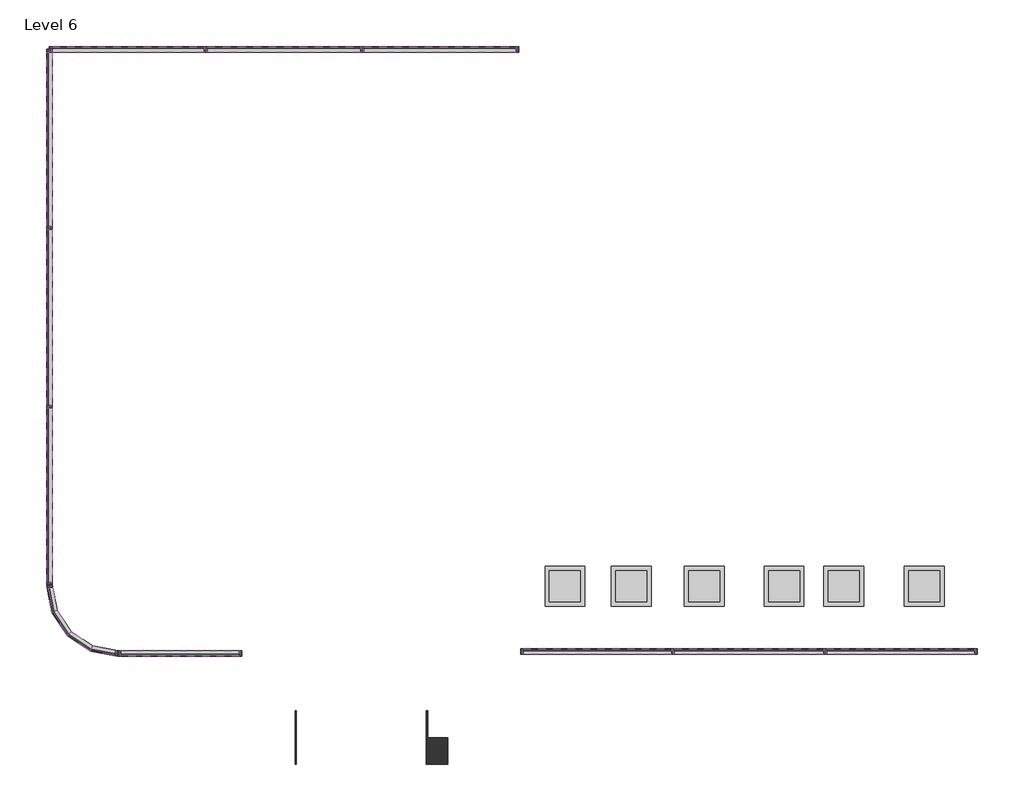
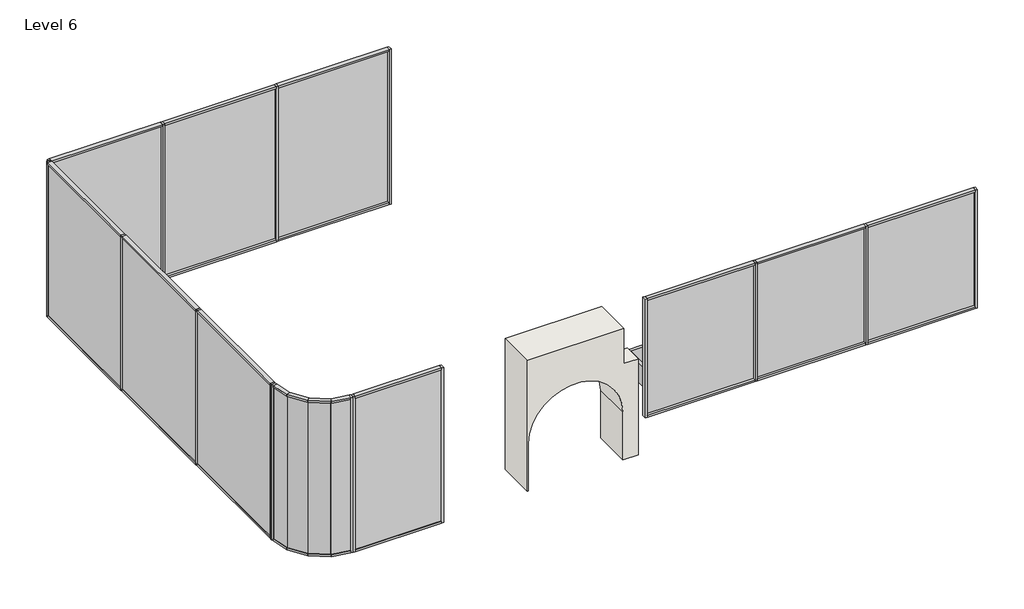
# One storey, incomplete: 44 members, 14 plates, 6 geographic elements, 1 wall.
"""IFC4 building model written with IfcOpenShell, lengths in millimetres."""

from ifc_helpers import new_model, si_unit, frame, origin, place, context, project, spatial, polyline, circle_curve, transform, mapped, element, save
from ifc_brep_helpers import plane_surface, revolved_surface, advanced_brep
from components import geographic_element_4c884dac, member_e5c989f4, member_5be86ab4, member_c6c1cc64, member_e826b105, member_eb03db27, member_3a1e0d67, member_7582bdd1, member_49f7f43a, member_78a27e2d, member_6a95fd14, member_1706ff29, member_70a47126, member_8659189c, member_4115b715, system_panel_glazed_8a9794be, system_panel_glazed_b9555dd7, system_panel_glazed_2aedba99, system_panel_glazed_5cb243be, system_panel_glazed_83a6671e, system_panel_glazed_ccff25ac, system_panel_glazed_ecbfc98a, system_panel_glazed_8a9bbf22, system_panel_glazed_1ec048b2

model = new_model("IFC4")

# Units and contexts
model_context = context("Model", 3, world=origin())
ifc_project = project(units=[si_unit("LENGTHUNIT", "METRE", prefix="MILLI")], contexts=[model_context])

# Site, building, storey
site = spatial("IfcSite", under=ifc_project)
building = spatial("IfcBuilding", under=site)
storey = spatial("IfcBuildingStorey", under=building, Name="Level 6", Elevation=12192.0)

# Geographic elements
placement = place(None, origin())
geographic_element_shape = geographic_element_4c884dac(model_context)
element("IfcGeographicElement", 1, ObjectType="Planter : 36\" x 36\"", at=placement, inside=storey, context=model_context, shape_type="MappedRepresentation", body=[
    mapped(geographic_element_shape, transform((3263.6150045, -1527.9908042, 11277.6), x_axis=(1.0, 0.0, 0.0), y_axis=(0.0, 1.0, 0.0), z_axis=(0.0, 0.0, 1.0))),
])
element("IfcGeographicElement", 2, ObjectType="Planter : 36\" x 36\"", at=placement, inside=storey, context=model_context, shape_type="MappedRepresentation", body=[
    mapped(geographic_element_shape, transform((1413.563121, -1527.9908042, 11277.6), x_axis=(1.0, 0.0, 0.0), y_axis=(0.0, 1.0, 0.0), z_axis=(0.0, 0.0, 1.0))),
])
element("IfcGeographicElement", 3, ObjectType="Planter : 36\" x 36\"", at=placement, inside=storey, context=model_context, shape_type="MappedRepresentation", body=[
    mapped(geographic_element_shape, transform((41.963121, -1527.9908042, 11277.6), x_axis=(1.0, 0.0, 0.0), y_axis=(0.0, 1.0, 0.0), z_axis=(0.0, 0.0, 1.0))),
])
element("IfcGeographicElement", 4, ObjectType="Planter : 36\" x 36\"", at=placement, inside=storey, context=model_context, shape_type="MappedRepresentation", body=[
    mapped(geographic_element_shape, transform((-1786.836879, -1527.9908042, 11277.6), x_axis=(1.0, 0.0, 0.0), y_axis=(0.0, 1.0, 0.0), z_axis=(0.0, 0.0, 1.0))),
])
element("IfcGeographicElement", 5, ObjectType="Planter : 36\" x 36\"", at=placement, inside=storey, context=model_context, shape_type="MappedRepresentation", body=[
    mapped(geographic_element_shape, transform((-3463.236879, -1527.9908042, 11277.6), x_axis=(1.0, 0.0, 0.0), y_axis=(0.0, 1.0, 0.0), z_axis=(0.0, 0.0, 1.0))),
])
element("IfcGeographicElement", 6, ObjectType="Planter : 36\" x 36\"", at=placement, inside=storey, context=model_context, shape_type="MappedRepresentation", body=[
    mapped(geographic_element_shape, transform((-4987.236879, -1527.9908042, 11277.6), x_axis=(1.0, 0.0, 0.0), y_axis=(0.0, 1.0, 0.0), z_axis=(0.0, 0.0, 1.0))),
])

# Members
member_shape = member_e5c989f4(model_context)
element("IfcMember", 7, ObjectType="Rectangular Mullion : 2.5\" x 5\" rectangular", at=placement, inside=storey, context=model_context, shape_type="MappedRepresentation", body=[
    mapped(member_shape, transform((-2507.8862511, -3028.3602909, 11201.4), x_axis=(1.0, 0.0, 0.0), y_axis=(0.0, -1.0, 0.0), z_axis=(0.0, 0.0, -1.0))),
])
element("IfcMember", 8, ObjectType="Rectangular Mullion : 2.5\" x 5\" rectangular", at=placement, inside=storey, context=model_context, shape_type="MappedRepresentation", body=[
    mapped(member_shape, transform((987.4643767, -3028.3602909, 11201.4), x_axis=(1.0, 0.0, 0.0), y_axis=(0.0, -1.0, 0.0), z_axis=(0.0, 0.0, -1.0))),
])
member_2_shape = member_5be86ab4(model_context)
element("IfcMember", 9, ObjectType="Rectangular Mullion : 2.5\" x 5\" rectangular", at=placement, inside=storey, context=model_context, shape_type="MappedRepresentation", body=[
    mapped(member_2_shape, transform((4482.8150045, -3028.3602909, 11201.4), x_axis=(1.0, 0.0, 0.0), y_axis=(0.0, -1.0, 0.0), z_axis=(0.0, 0.0, -1.0))),
])
element("IfcMember", 10, ObjectType="Rectangular Mullion : 2.5\" x 5\" rectangular", at=placement, inside=storey, context=model_context, shape_type="MappedRepresentation", body=[
    mapped(member_2_shape, transform((-6003.236879, -3028.3602909, 15163.8), x_axis=(-1.0, 0.0, 0.0), y_axis=(0.0, -1.0, 0.0), z_axis=(0.0, 0.0, 1.0))),
])
member_3_shape = member_c6c1cc64(model_context)
element("IfcMember", 11, ObjectType="Rectangular Mullion : 2.5\" x 5\" rectangular", at=placement, inside=storey, context=model_context, shape_type="MappedRepresentation", body=[
    mapped(member_3_shape, transform((-16364.0705833, -2617.2153653, 9982.2), x_axis=(0.0, 0.0, -1.0), y_axis=(0.8314696123025538, 0.5555702330195895, 0.0), z_axis=(0.5555702330195895, -0.8314696123025538, 0.0))),
])
element("IfcMember", 12, ObjectType="Rectangular Mullion : 2.5\" x 5\" rectangular", at=placement, inside=storey, context=model_context, shape_type="MappedRepresentation", body=[
    mapped(member_3_shape, transform((-16705.9599342, -2105.5417925, 15163.8), x_axis=(0.0, 0.0, 1.0), y_axis=(0.8314696123025543, 0.5555702330195887, 0.0), z_axis=(-0.5555702330195886, 0.8314696123025542, 0.0))),
])
element("IfcMember", 13, ObjectType="Rectangular Mullion : 2.5\" x 5\" rectangular", at=placement, inside=storey, context=model_context, shape_type="MappedRepresentation", body=[
    mapped(member_3_shape, transform((-16364.0705833, -2617.2153653, 15163.8), x_axis=(0.0, 0.0, 1.0), y_axis=(0.5555702330196195, 0.8314696123025337, 0.0), z_axis=(-0.8314696123025337, 0.5555702330196195, 0.0))),
])
element("IfcMember", 14, ObjectType="Rectangular Mullion : 2.5\" x 5\" rectangular", at=placement, inside=storey, context=model_context, shape_type="MappedRepresentation", body=[
    mapped(member_3_shape, transform((-15852.3970105, -2959.1047162, 9982.2), x_axis=(0.0, 0.0, -1.0), y_axis=(0.5555702330196192, 0.831469612302534, 0.0), z_axis=(0.8314696123025339, -0.555570233019619, 0.0))),
])
member_4_shape = member_e826b105(model_context)
element("IfcMember", 15, ObjectType="Rectangular Mullion : 2.5\" x 5\" rectangular", at=placement, inside=storey, context=model_context, shape_type="MappedRepresentation", body=[
    mapped(member_4_shape, transform((-15185.336879, -3079.1602909, 15163.8), x_axis=(0.0, 0.0, 1.0), y_axis=(0.0, 1.0, 0.0), z_axis=(-1.0, 0.0, 0.0))),
])
element("IfcMember", 16, ObjectType="Rectangular Mullion : 2.5\" x 5\" rectangular", at=placement, inside=storey, context=model_context, shape_type="MappedRepresentation", body=[
    mapped(member_4_shape, transform((-12467.536879, -3079.1602909, 9982.2), x_axis=(0.0, 0.0, -1.0), y_axis=(0.0, 1.0, 0.0), z_axis=(1.0, 0.0, 0.0))),
])
member_5_shape = member_eb03db27(model_context)
element("IfcMember", 17, ObjectType="Rectangular Mullion : 2.5\" x 5\" rectangular", at=placement, inside=storey, context=model_context, shape_type="MappedRepresentation", body=[
    mapped(member_5_shape, transform((-6108.1002522, 10795.6437739, 15163.8), x_axis=(0.0, 0.0, 1.0), y_axis=(0.0, -1.0, 0.0), z_axis=(1.0, 0.0, 0.0))),
])
element("IfcMember", 18, ObjectType="Rectangular Mullion : 2.5\" x 5\" rectangular", at=placement, inside=storey, context=model_context, shape_type="MappedRepresentation", body=[
    mapped(member_5_shape, transform((-13263.9604233, 10795.6437739, 15163.8), x_axis=(0.0, 0.0, 1.0), y_axis=(0.0, -1.0, 0.0), z_axis=(1.0, 0.0, 0.0))),
])
member_6_shape = member_3a1e0d67(model_context)
element("IfcMember", 19, ObjectType="Rectangular Mullion : 2.5\" x 5\" rectangular", at=placement, inside=storey, context=model_context, shape_type="MappedRepresentation", body=[
    mapped(member_6_shape, transform((-9670.1553377, 10795.6437739, 15163.8), x_axis=(0.0, 0.0, 1.0), y_axis=(0.0, -1.0, 0.0), z_axis=(1.0, 0.0, 0.0))),
])
element("IfcMember", 20, ObjectType="Rectangular Mullion : 2.5\" x 5\" rectangular", at=placement, inside=storey, context=model_context, shape_type="MappedRepresentation", body=[
    mapped(member_5_shape, transform((-16762.5155088, 10795.6437739, 9982.2), x_axis=(0.0, 0.0, -1.0), y_axis=(0.0, -1.0, 0.0), z_axis=(-1.0, 0.0, 0.0))),
])
element("IfcMember", 21, ObjectType="Rectangular Mullion : 2.5\" x 5\" rectangular", at=placement, inside=storey, context=model_context, shape_type="MappedRepresentation", body=[
    mapped(member_5_shape, transform((-9606.6553377, 10795.6437739, 9982.2), x_axis=(0.0, 0.0, -1.0), y_axis=(0.0, -1.0, 0.0), z_axis=(-1.0, 0.0, 0.0))),
])
element("IfcMember", 22, ObjectType="Rectangular Mullion : 2.5\" x 5\" rectangular", at=placement, inside=storey, context=model_context, shape_type="MappedRepresentation", body=[
    mapped(member_6_shape, transform((-13200.4604233, 10795.6437739, 9982.2), x_axis=(0.0, 0.0, -1.0), y_axis=(0.0, -1.0, 0.0), z_axis=(-1.0, 0.0, 0.0))),
])
member_7_shape = member_7582bdd1(model_context)
element("IfcMember", 23, ObjectType="Rectangular Mullion : 2.5\" x 5\" rectangular", at=placement, inside=storey, context=model_context, shape_type="MappedRepresentation", body=[
    mapped(member_7_shape, transform((-16826.0155088, 10732.1437739, 15163.8), x_axis=(0.0, 0.0, 1.0), y_axis=(1.0, 0.0, 0.0), z_axis=(0.0, 1.0, 0.0))),
])
element("IfcMember", 24, ObjectType="Rectangular Mullion : 2.5\" x 5\" rectangular", at=placement, inside=storey, context=model_context, shape_type="MappedRepresentation", body=[
    mapped(member_7_shape, transform((-16826.0155088, 2565.4768173, 15163.8), x_axis=(0.0, 0.0, 1.0), y_axis=(1.0, 0.0, 0.0), z_axis=(0.0, 1.0, 0.0))),
])
member_8_shape = member_49f7f43a(model_context)
element("IfcMember", 25, ObjectType="Rectangular Mullion : 2.5\" x 5\" rectangular", at=placement, inside=storey, context=model_context, shape_type="MappedRepresentation", body=[
    mapped(member_8_shape, transform((-16826.0155088, 6664.6852956, 15163.8), x_axis=(0.0, 0.0, 1.0), y_axis=(1.0, 0.0, 0.0), z_axis=(0.0, 1.0, 0.0))),
])
element("IfcMember", 26, ObjectType="Rectangular Mullion : 2.5\" x 5\" rectangular", at=placement, inside=storey, context=model_context, shape_type="MappedRepresentation", body=[
    mapped(member_7_shape, transform((-16826.0155088, -1438.481661, 9982.2), x_axis=(0.0, 0.0, -1.0), y_axis=(1.0, 0.0, 0.0), z_axis=(0.0, -1.0, 0.0))),
])
element("IfcMember", 27, ObjectType="Rectangular Mullion : 2.5\" x 5\" rectangular", at=placement, inside=storey, context=model_context, shape_type="MappedRepresentation", body=[
    mapped(member_7_shape, transform((-16826.0155088, 6728.1852956, 9982.2), x_axis=(0.0, 0.0, -1.0), y_axis=(1.0, 0.0, 0.0), z_axis=(0.0, -1.0, 0.0))),
])
element("IfcMember", 28, ObjectType="Rectangular Mullion : 2.5\" x 5\" rectangular", at=placement, inside=storey, context=model_context, shape_type="MappedRepresentation", body=[
    mapped(member_8_shape, transform((-16826.0155088, 2628.9768173, 9982.2), x_axis=(0.0, 0.0, -1.0), y_axis=(1.0, 0.0, 0.0), z_axis=(0.0, -1.0, 0.0))),
])
member_9_shape = member_78a27e2d(model_context)
element("IfcMember", 29, ObjectType="Rectangular Mullion : 2.5\" x 5\" rectangular", at=placement, inside=storey, context=model_context, shape_type="MappedRepresentation", body=[
    mapped(member_9_shape, transform((4419.3150045, -3028.3602909, 15163.8), x_axis=(0.0, 0.0, 1.0), y_axis=(0.0, -1.0, 0.0), z_axis=(1.0, 0.0, 0.0))),
])
element("IfcMember", 30, ObjectType="Rectangular Mullion : 2.5\" x 5\" rectangular", at=placement, inside=storey, context=model_context, shape_type="MappedRepresentation", body=[
    mapped(member_9_shape, transform((-2539.6362511, -3028.3602909, 15163.8), x_axis=(0.0, 0.0, 1.0), y_axis=(0.0, -1.0, 0.0), z_axis=(1.0, 0.0, 0.0))),
])
member_10_shape = member_6a95fd14(model_context)
element("IfcMember", 31, ObjectType="Rectangular Mullion : 2.5\" x 5\" rectangular", at=placement, inside=storey, context=model_context, shape_type="MappedRepresentation", body=[
    mapped(member_10_shape, transform((955.7143767, -3028.3602909, 15163.8), x_axis=(0.0, 0.0, 1.0), y_axis=(0.0, -1.0, 0.0), z_axis=(1.0, 0.0, 0.0))),
])
element("IfcMember", 32, ObjectType="Rectangular Mullion : 2.5\" x 5\" rectangular", at=placement, inside=storey, context=model_context, shape_type="MappedRepresentation", body=[
    mapped(member_9_shape, transform((-5939.736879, -3028.3602909, 11201.4), x_axis=(0.0, 0.0, -1.0), y_axis=(0.0, -1.0, 0.0), z_axis=(-1.0, 0.0, 0.0))),
])
element("IfcMember", 33, ObjectType="Rectangular Mullion : 2.5\" x 5\" rectangular", at=placement, inside=storey, context=model_context, shape_type="MappedRepresentation", body=[
    mapped(member_9_shape, transform((1019.2143767, -3028.3602909, 11201.4), x_axis=(0.0, 0.0, -1.0), y_axis=(0.0, -1.0, 0.0), z_axis=(-1.0, 0.0, 0.0))),
])
element("IfcMember", 34, ObjectType="Rectangular Mullion : 2.5\" x 5\" rectangular", at=placement, inside=storey, context=model_context, shape_type="MappedRepresentation", body=[
    mapped(member_10_shape, transform((-2476.1362511, -3028.3602909, 11201.4), x_axis=(0.0, 0.0, -1.0), y_axis=(0.0, -1.0, 0.0), z_axis=(-1.0, 0.0, 0.0))),
])
member_11_shape = member_1706ff29(model_context)
element("IfcMember", 35, ObjectType="Rectangular Mullion : 2.5\" x 5\" rectangular", at=placement, inside=storey, context=model_context, shape_type="MappedRepresentation", body=[
    mapped(member_11_shape, transform((-16826.0155088, 2597.2268173, 9982.2), x_axis=(0.0, 1.0, 0.0), y_axis=(1.0, 0.0, 0.0), z_axis=(0.0, 0.0, -1.0))),
])
element("IfcMember", 36, ObjectType="Rectangular Mullion : 2.5\" x 5\" rectangular", at=placement, inside=storey, context=model_context, shape_type="MappedRepresentation", body=[
    mapped(member_11_shape, transform((-16826.0155088, 6696.4352956, 9982.2), x_axis=(0.0, 1.0, 0.0), y_axis=(1.0, 0.0, 0.0), z_axis=(0.0, 0.0, -1.0))),
])
element("IfcMember", 37, ObjectType="Rectangular Mullion : 2.5\" x 5\" rectangular", at=placement, inside=storey, context=model_context, shape_type="MappedRepresentation", body=[
    mapped(member_11_shape, transform((-13232.2104233, 10795.6437739, 9982.2), x_axis=(1.0, 0.0, 0.0), y_axis=(0.0, -1.0, 0.0), z_axis=(0.0, 0.0, -1.0))),
])
element("IfcMember", 38, ObjectType="Rectangular Mullion : 2.5\" x 5\" rectangular", at=placement, inside=storey, context=model_context, shape_type="MappedRepresentation", body=[
    mapped(member_11_shape, transform((-9638.4053377, 10795.6437739, 9982.2), x_axis=(1.0, 0.0, 0.0), y_axis=(0.0, -1.0, 0.0), z_axis=(0.0, 0.0, -1.0))),
])
member_12_shape = member_70a47126(model_context)
element("IfcMember", 39, ObjectType="Rectangular Mullion : 2.5\" x 5\" rectangular", at=placement, inside=storey, context=model_context, shape_type="MappedRepresentation", body=[
    mapped(member_12_shape, transform((-15248.836879, -3079.1602909, 9982.2), x_axis=(-1.0, 0.0, 0.0), y_axis=(0.0, 1.0, 0.0), z_axis=(0.0, 0.0, -1.0))),
])
element("IfcMember", 40, ObjectType="Rectangular Mullion : 2.5\" x 5\" rectangular", at=placement, inside=storey, context=model_context, shape_type="MappedRepresentation", body=[
    mapped(member_12_shape, transform((-16826.0155088, -1501.981661, 9982.2), x_axis=(-0.19509032201611803, 0.9807852804032325, 0.0), y_axis=(0.9807852804032325, 0.19509032201611803, 0.0), z_axis=(0.0, 0.0, -1.0))),
])
element("IfcMember", 41, ObjectType="Rectangular Mullion : 2.5\" x 5\" rectangular", at=placement, inside=storey, context=model_context, shape_type="MappedRepresentation", body=[
    mapped(member_12_shape, transform((-16826.0155088, 10795.6437739, 9982.2), x_axis=(0.0, 1.0, 0.0), y_axis=(1.0, 0.0, 0.0), z_axis=(0.0, 0.0, -1.0))),
])
element("IfcMember", 42, ObjectType="Rectangular Mullion : 2.5\" x 5\" rectangular", at=placement, inside=storey, context=model_context, shape_type="MappedRepresentation", body=[
    mapped(member_12_shape, transform((-6044.6002522, 10795.6437739, 9982.2), x_axis=(1.0, 0.0, 0.0), y_axis=(0.0, -1.0, 0.0), z_axis=(0.0, 0.0, -1.0))),
])
element("IfcMember", 43, ObjectType="Rectangular Mullion : 2.5\" x 5\" rectangular", at=placement, inside=storey, context=model_context, shape_type="MappedRepresentation", body=[
    mapped(member_12_shape, transform((-12404.036879, -3079.1602909, 15163.8), x_axis=(1.0, 0.0, 0.0), y_axis=(0.0, 1.0, 0.0), z_axis=(0.0, 0.0, 1.0))),
])
element("IfcMember", 44, ObjectType="Rectangular Mullion : 2.5\" x 5\" rectangular", at=placement, inside=storey, context=model_context, shape_type="MappedRepresentation", body=[
    mapped(member_12_shape, transform((-15248.836879, -3079.1602909, 15163.8), x_axis=(0.9807852804032272, -0.1950903220161449, 0.0), y_axis=(0.1950903220161449, 0.9807852804032272, 0.0), z_axis=(0.0, 0.0, 1.0))),
])
element("IfcMember", 45, ObjectType="Rectangular Mullion : 2.5\" x 5\" rectangular", at=placement, inside=storey, context=model_context, shape_type="MappedRepresentation", body=[
    mapped(member_12_shape, transform((-16826.0155088, -1501.981661, 15163.8), x_axis=(0.0, -1.0, 0.0), y_axis=(1.0, 0.0, 0.0), z_axis=(0.0, 0.0, 1.0))),
])
element("IfcMember", 46, ObjectType="Rectangular Mullion : 2.5\" x 5\" rectangular", at=placement, inside=storey, context=model_context, shape_type="MappedRepresentation", body=[
    mapped(member_12_shape, transform((-16826.0155088, 10795.6437739, 15163.8), x_axis=(-1.0, 0.0, 0.0), y_axis=(0.0, -1.0, 0.0), z_axis=(0.0, 0.0, 1.0))),
])
member_13_shape = member_8659189c(model_context)
element("IfcMember", 47, ObjectType="Rectangular Mullion : 2.5\" x 5\" rectangular", at=placement, inside=storey, context=model_context, shape_type="MappedRepresentation", body=[
    mapped(member_13_shape, transform((-16813.6272734, -1564.2615263, 15163.8), x_axis=(0.0, 0.0, 1.0), y_axis=(0.9807852804032325, 0.195090322016118, 0.0), z_axis=(-0.195090322016118, 0.9807852804032325, 0.0))),
])
element("IfcMember", 48, ObjectType="Rectangular Mullion : 2.5\" x 5\" rectangular", at=placement, inside=storey, context=model_context, shape_type="MappedRepresentation", body=[
    mapped(member_13_shape, transform((-15311.1167443, -3066.7720554, 9982.2), x_axis=(0.0, 0.0, -1.0), y_axis=(0.1950903220161449, 0.9807852804032272, 0.0), z_axis=(0.9807852804032271, -0.19509032201614487, 0.0))),
])
member_14_shape = member_4115b715(model_context)
element("IfcMember", 49, ObjectType="Rectangular Mullion : 2.5\" x 5\" rectangular", at=placement, inside=storey, context=model_context, shape_type="MappedRepresentation", body=[
    mapped(member_14_shape, transform((-16705.9599342, -2105.5417925, 9982.2), x_axis=(0.0, 0.0, -1.0), y_axis=(0.9807852804032325, 0.195090322016118, 0.0), z_axis=(0.195090322016118, -0.9807852804032325, 0.0))),
])
element("IfcMember", 50, ObjectType="Rectangular Mullion : 2.5\" x 5\" rectangular", at=placement, inside=storey, context=model_context, shape_type="MappedRepresentation", body=[
    mapped(member_14_shape, transform((-15852.3970105, -2959.1047162, 15163.8), x_axis=(0.0, 0.0, 1.0), y_axis=(0.1950903220161449, 0.9807852804032272, 0.0), z_axis=(-0.9807852804032271, 0.19509032201614487, 0.0))),
])

# Plates
system_panel_glazed_shape = system_panel_glazed_8a9794be(model_context)
element("IfcPlate", 51, ObjectType="System Panel : Glazed", at=placement, inside=storey, context=model_context, shape_type="MappedRepresentation", body=[
    mapped(system_panel_glazed_shape, transform((-4239.6865651, -3028.3602909, 11264.9), x_axis=(1.0, 0.0, 0.0), y_axis=(0.0, 1.0, 0.0), z_axis=(0.0, 0.0, 1.0))),
])
element("IfcPlate", 52, ObjectType="System Panel : Glazed", at=placement, inside=storey, context=model_context, shape_type="MappedRepresentation", body=[
    mapped(system_panel_glazed_shape, transform((2719.2646906, -3028.3602909, 11264.9), x_axis=(1.0, 0.0, 0.0), y_axis=(0.0, 1.0, 0.0), z_axis=(0.0, 0.0, 1.0))),
])
system_panel_glazed_2_shape = system_panel_glazed_b9555dd7(model_context)
element("IfcPlate", 53, ObjectType="System Panel : Glazed", at=placement, inside=storey, context=model_context, shape_type="MappedRepresentation", body=[
    mapped(system_panel_glazed_2_shape, transform((-760.2109372, -3028.3602909, 11264.9), x_axis=(1.0, 0.0, 0.0), y_axis=(0.0, 1.0, 0.0), z_axis=(0.0, 0.0, 1.0))),
])
system_panel_glazed_3_shape = system_panel_glazed_2aedba99(model_context)
element("IfcPlate", 54, ObjectType="System Panel : Glazed", at=placement, inside=storey, context=model_context, shape_type="MappedRepresentation", body=[
    mapped(system_panel_glazed_3_shape, transform((-15013.237966, 10795.6437739, 10045.7), x_axis=(1.0, 0.0, 0.0), y_axis=(0.0, 1.0, 0.0), z_axis=(0.0, 0.0, 1.0))),
])
element("IfcPlate", 55, ObjectType="System Panel : Glazed", at=placement, inside=storey, context=model_context, shape_type="MappedRepresentation", body=[
    mapped(system_panel_glazed_3_shape, transform((-7857.3777949, 10795.6437739, 10045.7), x_axis=(1.0, 0.0, 0.0), y_axis=(0.0, 1.0, 0.0), z_axis=(0.0, 0.0, 1.0))),
])
system_panel_glazed_4_shape = system_panel_glazed_5cb243be(model_context)
element("IfcPlate", 56, ObjectType="System Panel : Glazed", at=placement, inside=storey, context=model_context, shape_type="MappedRepresentation", body=[
    mapped(system_panel_glazed_4_shape, transform((-11435.3078805, 10795.6437739, 10045.7), x_axis=(1.0, 0.0, 0.0), y_axis=(0.0, 1.0, 0.0), z_axis=(0.0, 0.0, 1.0))),
])
system_panel_glazed_5_shape = system_panel_glazed_83a6671e(model_context)
element("IfcPlate", 57, ObjectType="System Panel : Glazed", at=placement, inside=storey, context=model_context, shape_type="MappedRepresentation", body=[
    mapped(system_panel_glazed_5_shape, transform((-16826.0155088, 563.4975781, 10045.7), x_axis=(0.0, 1.0, 0.0), y_axis=(-1.0, 0.0, 0.0), z_axis=(0.0, 0.0, 1.0))),
])
element("IfcPlate", 58, ObjectType="System Panel : Glazed", at=placement, inside=storey, context=model_context, shape_type="MappedRepresentation", body=[
    mapped(system_panel_glazed_5_shape, transform((-16826.0155088, 8730.1645348, 10045.7), x_axis=(0.0, 1.0, 0.0), y_axis=(-1.0, 0.0, 0.0), z_axis=(0.0, 0.0, 1.0))),
])
system_panel_glazed_6_shape = system_panel_glazed_ccff25ac(model_context)
element("IfcPlate", 59, ObjectType="System Panel : Glazed", at=placement, inside=storey, context=model_context, shape_type="MappedRepresentation", body=[
    mapped(system_panel_glazed_6_shape, transform((-16826.0155088, 4646.8310564, 10045.7), x_axis=(0.0, 1.0, 0.0), y_axis=(-1.0, 0.0, 0.0), z_axis=(0.0, 0.0, 1.0))),
])
system_panel_glazed_7_shape = system_panel_glazed_ecbfc98a(model_context)
element("IfcPlate", 60, ObjectType="System Panel : Glazed", at=placement, inside=storey, context=model_context, shape_type="MappedRepresentation", body=[
    mapped(system_panel_glazed_7_shape, transform((-15581.7568774, -3012.9383858, 10045.7), x_axis=(-0.9807852804032272, 0.19509032201614493, 0.0), y_axis=(-0.19509032201614493, -0.9807852804032272, 0.0), z_axis=(0.0, 0.0, 1.0))),
])
element("IfcPlate", 61, ObjectType="System Panel : Glazed", at=placement, inside=storey, context=model_context, shape_type="MappedRepresentation", body=[
    mapped(system_panel_glazed_7_shape, transform((-16759.7936038, -1834.9016594, 10045.7), x_axis=(-0.19509032201611803, 0.9807852804032325, 0.0), y_axis=(-0.9807852804032325, -0.19509032201611803, 0.0), z_axis=(0.0, 0.0, 1.0))),
])
system_panel_glazed_8_shape = system_panel_glazed_8a9bbf22(model_context)
element("IfcPlate", 62, ObjectType="System Panel : Glazed", at=placement, inside=storey, context=model_context, shape_type="MappedRepresentation", body=[
    mapped(system_panel_glazed_8_shape, transform((-16535.0152587, -2361.3785789, 10045.7), x_axis=(-0.5555702330195887, 0.8314696123025543, 0.0), y_axis=(-0.8314696123025543, -0.5555702330195887, 0.0), z_axis=(0.0, 0.0, 1.0))),
])
element("IfcPlate", 63, ObjectType="System Panel : Glazed", at=placement, inside=storey, context=model_context, shape_type="MappedRepresentation", body=[
    mapped(system_panel_glazed_8_shape, transform((-16108.2337969, -2788.1600408, 10045.7), x_axis=(-0.8314696123025337, 0.5555702330196195, 0.0), y_axis=(-0.5555702330196195, -0.8314696123025337, 0.0), z_axis=(0.0, 0.0, 1.0))),
])
system_panel_glazed_9_shape = system_panel_glazed_1ec048b2(model_context)
element("IfcPlate", 64, ObjectType="System Panel : Glazed", at=placement, inside=storey, context=model_context, shape_type="MappedRepresentation", body=[
    mapped(system_panel_glazed_9_shape, transform((-13826.436879, -3079.1602909, 10045.7), x_axis=(-1.0, 0.0, 0.0), y_axis=(0.0, -1.0, 0.0), z_axis=(0.0, 0.0, 1.0))),
])

# Wall
element("IfcWall", 65, ObjectType="Generic - 7'", at=placement, inside=storey, context=model_context, shape_type="AdvancedBrep", body=[
    advanced_brep(
    [(-8136.836879, -4394.9713144, 12090.4), (-8170.0615732, -4394.9713144, 12090.4), (-8170.0615732, -4394.9713144, 13673.1934663), (-11151.6121848, -4394.9713144, 13673.1934663), (-11151.6121848, -4394.9713144, 12090.4), (-11184.836879, -4394.9713144, 12090.4), (-11184.836879, -4394.9713144, 16459.2), (-8136.836879, -4394.9713144, 16459.2), (-8136.836879, -4394.9713144, 15290.8), (-7679.636879, -5614.1713144, 12090.4), (-7679.636879, -5614.1713144, 15290.8), (-8136.836879, -5614.1713144, 15290.8), (-8136.836879, -5614.1713144, 16455.5534623), (-8136.836879, -5614.1713144, 16459.2), (-11184.836879, -5614.1713144, 16459.2), (-11184.836879, -5614.1713144, 12090.4), (-11151.6121848, -5614.1713144, 12090.4), (-11151.6121848, -5614.1713144, 13673.1934663), (-8170.0615732, -5614.1713144, 13673.1934663), (-8170.0615732, -5614.1713144, 12090.4), (-8136.836879, -5004.5713144, 15290.8), (-8136.836879, -5004.5713144, 12090.4), (-7679.636879, -5004.5713144, 15290.8), (-7679.636879, -5004.5713144, 12090.4)],
    [
        (0, 1),
        (1, 2),
        (2, 3, circle_curve(frame((-9660.836879, -4394.9713144, 13673.1934663), z_axis=(0.0, -1.0, 0.0), x_axis=(1.0, 0.0, 0.0)), 1490.7753058)),
        (3, 4),
        (4, 5),
        (5, 6),
        (6, 7),
        (7, 8),
        (8, 0),
        (9, 10),
        (10, 11),
        (11, 12),
        (12, 13),
        (13, 14),
        (14, 15),
        (15, 16),
        (16, 17),
        (17, 18, circle_curve(frame((-9660.836879, -5614.1713144, 13673.1934663), z_axis=(0.0, 1.0, 0.0), x_axis=(1.0, 0.0, 0.0)), 1490.7753058)),
        (18, 19),
        (19, 9),
        (8, 20),
        (20, 21),
        (21, 0),
        (7, 13),
        (11, 20),
        (5, 15),
        (14, 6),
        (10, 22),
        (22, 20),
        (22, 23),
        (23, 21),
        (9, 23),
        (19, 1),
        (18, 2),
        (17, 3),
        (16, 4),
    ],
    [
        plane_surface(frame((-8170.0615732, -4394.9713144, 12090.4), z_axis=(0.0, 1.0, 0.0), x_axis=(-1.0, 0.0, 0.0))),
        plane_surface(frame((-8170.0615732, -5614.1713144, 12090.4), z_axis=(0.0, -1.0, 0.0), x_axis=(1.0, 0.0, 0.0))),
        plane_surface(frame((-8136.836879, -2870.9713144, 11871.96), z_axis=(1.0, 0.0, 0.0), x_axis=(0.0, 1.0, 0.0))),
        plane_surface(frame((-8136.836879, -3051.9908042, 5994.4), z_axis=(1.0, 0.0, 0.0), x_axis=(0.0, -1.0, 0.0))),
        plane_surface(frame((-11184.836879, -3051.9908042, 5994.4), z_axis=(-1.0, 0.0, 0.0), x_axis=(0.0, 1.0, 0.0))),
        plane_surface(frame((-11794.436879, -4394.9713144, 16459.2), z_axis=(0.0, 0.0, 1.0), x_axis=(0.0, -1.0, 0.0))),
        plane_surface(frame((-7527.236879, -4394.9713144, 15290.8), z_axis=(0.0, 0.0, 1.0), x_axis=(1.0, 0.0, 0.0))),
        plane_surface(frame((-7908.236879, -5004.5713144, 11871.96), z_axis=(0.0, 1.0, 0.0), x_axis=(-1.0, 0.0, 0.0))),
        plane_surface(frame((-7679.636879, -7138.1713144, 11871.96), z_axis=(1.0, 0.0, 0.0), x_axis=(0.0, 1.0, 0.0))),
        plane_surface(frame((-7527.236879, -4394.9713144, 12090.4), z_axis=(0.0, 0.0, -1.0), x_axis=(0.0, -1.0, 0.0))),
        plane_surface(frame((-8170.0615732, -4394.9713144, 12090.4), z_axis=(-1.0, 0.0, 0.0), x_axis=(0.0, -1.0, 0.0))),
        revolved_surface(polyline([(-8170.061573200001, -5614.1713144, 13673.1934663), (-8170.061573200001, -4394.9713144, 13673.1934663)]), (-9660.836879, -5614.1713144, 13673.1934663), (0.0, -1.0, 0.0)),
        plane_surface(frame((-11151.6121848, -4394.9713144, 13673.1934663), z_axis=(1.0, 0.0, 0.0), x_axis=(0.0, -1.0, 0.0))),
        plane_surface(frame((-11151.6121848, -4394.9713144, 12090.4), z_axis=(0.0, 0.0, -1.0), x_axis=(0.0, -1.0, 0.0))),
    ],
    [
        (0, [[1, 2, 3, 4, 5, 6, 7, 8, 9]]),
        (1, [[10, 11, 12, 13, 14, 15, 16, 17, 18, 19, 20]]),
        (2, [[-9, 21, 22, 23]]),
        (3, [[-8, 24, -13, -12, 25, -21]]),
        (4, [[-6, 26, -15, 27]]),
        (5, [[-7, -27, -14, -24]]),
        (6, [[-25, -11, 28, 29]]),
        (7, [[-29, 30, 31, -22]]),
        (8, [[-28, -10, 32, -30]]),
        (9, [[-1, -23, -31, -32, -20, 33]]),
        (10, [[-2, -33, -19, 34]]),
        (11, [[-3, -34, -18, 35]]),
        (12, [[-4, -35, -17, 36]]),
        (13, [[-5, -36, -16, -26]]),
    ],
),
])

save(model, "model.ifc")

# Revit data of these elements
# Type "Planter : 36\" x 36\""
#   Depth = 3' - 0"
#   Height = 2' - 6"
#   Width = 3' - 0"
#   Material = Concrete, Precast
# Type "Rectangular Mullion : 2.5\" x 5\" rectangular"
#   built-in parameter 1007304 = 0.416667 (stored number, unit not read)
#   built-in parameter 1007301 = 0.104167 (stored number, unit not read)
#   built-in parameter 1007300 = 0.104167 (stored number, unit not read)
# Type "System Panel : Glazed"
#   Construction Type Id = "GSP4R"
#   Analytic Construction = "1/8 in Pilkington single glazing"
#   Visual Light Transmittance = 0.9
#   Solar Heat Gain Coefficient = 0.86
#   Heat Transfer Coefficient (U) = 1.18115 BTU/(h·ft²·°F)
# Type "Generic - 7'"
#   Assembly Code = "B2010"
#   Layers, outside or top first: 4' - 0" "Parking Stripe" (function 1)
# Elements 1, 2, 3, 4, 5, 6 (IfcGeographicElement, "Planter : 36\" x 36\"")
#   Phase Created = New Construction
#   Materials on its faces: "Concrete, Precast"
# Elements 7, 8, 9, 10, 11, 12, 13, 14, 15, 16, 17, 18, 19, 20, 21, 22, 23, 24, 25, 26, 27, 28, 29, 30, 31, 32, 33, 34, 35, 36, 37, 38, 39, 40, 41, 42, 43, 44, 45, 46, 47, 48, 49, 50 (IfcMember, "Rectangular Mullion : 2.5\" x 5\" rectangular")
#   Phase Created = New Construction
#   Materials on its faces: "Iron, Ductile"
# Elements 51, 52, 53, 54, 55, 56, 57, 58, 59, 60, 61, 62, 63, 64 (IfcPlate, "System Panel : Glazed")
#   Phase Created = New Construction
#   Materials on its faces: "Glass"
# Element 65 (IfcWall, "Generic - 7'")
#   built-in parameter 1001111 = -0' - 4"
#   Top Offset = 0' - 0"
#   Base Offset = -0' - 4"
#   Unconnected Height = 14' - 4"
#   wall height = 14' - 4"
#   Phase Created = New Construction
#   Base Constraint = Level 6
#   Materials on its faces: "Parking Stripe"
# Materials
#   "Concrete, Precast": class "Concrete", colour RGB 198 187 187, transparency 0, Description = "Precast concrete", Cost = 0
#   "Parking Stripe": class "Paint", colour RGB 250 250 91, transparency 0, Cost = 0
#   "Iron, Ductile": class "Metal", colour RGB 0 0 0, transparency 0, Description = "Ductile cast iron", Cost = 0
#   "Glass": class "Glass", colour RGB 0 128 192, transparency 0.75, Description = "Soda Lime Glass", Cost = 0
